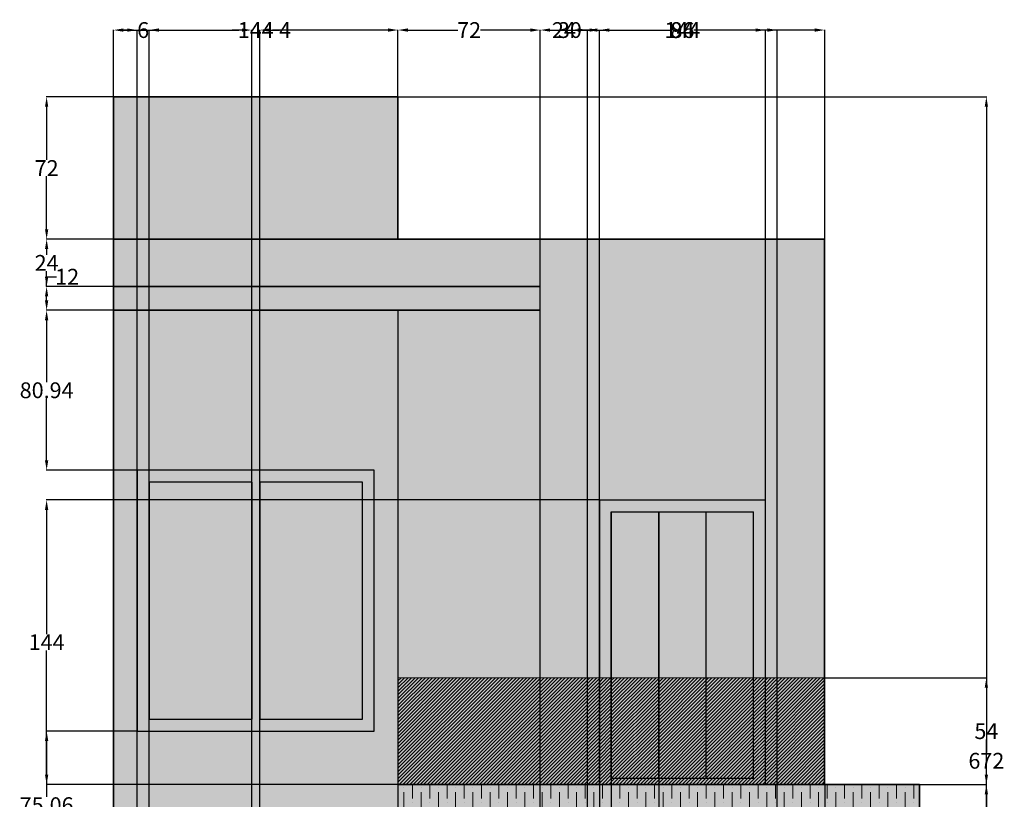
# Model space of a CAD drawing. Units: inches. Extents: x 137 to 641, y 88 to 838.
# Tile 2 of 2: x 142 to 641, y 444 to 838. Entities that reach past the tile are written whole.
import ezdxf

# ---------------------------------------------------------------- set-up
doc = ezdxf.new("R2010")
doc.units = ezdxf.units.IN
doc.header["$MEASUREMENT"] = 0
doc.layers.get('0').update_dxf_attribs({"color": 250})
for name, color, linetype, lineweight in [('A-ANNO-DIMS', 2, 'Continuous', 18), ('A-ELEV-TRIM-PATT', 18, 'Continuous', 13), ('A-FLOR-BALC', 250, 'Continuous', 35), ('A-FLOR-BALC-PATT', 250, 'Continuous', 13), ('A-FLOR-RAIL', 250, 'Continuous', 18), ('A-GLAZ', 250, 'Continuous', 25), ('A-GLAZ-PATT', 250, 'Continuous', 13), ('A-ROOF', 250, 'Continuous', 35), ('A-WALL', 250, 'Continuous', 35), ('A-WALL-CLAD', 250, 'Continuous', 25)]:
    doc.layers.add(name, color=color, linetype=linetype, lineweight=lineweight)
for name, color, linetype, lineweight, true_color in [('A-FLOR-BALC-FILL', 89, 'Continuous', 13, 0x333e19), ('A-FLOR-RAIL-PATT', 251, 'Continuous', 13, 0x636466), ('A-ROOF-PATT', 250, 'Continuous', 13, 0x303030), ('A-WALL-CLAD-FILL', 51, 'Continuous', 13, 0xfff4a4), ('A-WALL-CLAD-PATT', 21, 'Continuous', 13, 0xe2a688), ('A-WALL-PATT', 254, 'Continuous', 13, 0xd7ebd2)]:
    doc.layers.add(name, color=color, linetype=linetype, lineweight=lineweight, true_color=true_color)
doc.styles.get("Standard").update_dxf_attribs({"font": 'arial.ttf'})
doc.dimstyles.get("Standard").update_dxf_attribs({"dimtxt": 8, "dimasz": 5, "dimexe": 0.18, "dimexo": 0.0625, "dimgap": 0.09, "dimtad": 0, "dimtih": 1, "dimtoh": 1, "dimdec": 0, "dimzin": 0, "dimdsep": 46, "dimlunit": 3, "dimtxsty": 'Standard', "dimcen": 0.09, "dimadec": 0, "dimazin": 0, "dimtfac": 1, "dimtdec": 0, "dimtofl": 0, "dimtmove": 0, "dimatfit": 3, "dimfxl": 1, "dimtolj": 1, "dimtzin": 0, "dimarcsym": 0})

# ---------------------------------------------------------------- blocks, each defined once
blk = doc.blocks.new('WIN-FRAME-2L-120X132')
for p, q in [((58, 126), (58, 6)), ((62, 126), (62, 6))]:
    blk.add_line(p, q)
for points in [[(120, 132), (0, 132)], [(0, 132), (0, 0), (120, 0), (120, 132)], [(58, 126), (6, 126)], [(6, 126), (6, 6), (58, 6)], [(62, 6), (114, 6), (114, 126)], [(114, 126), (62, 126)]]:
    blk.add_lwpolyline(points)
blk = doc.blocks.new('*D5')
at = {"layer": 'A-ANNO-DIMS', "color": 0, "lineweight": -2, "transparency": 16777216}
for p, q in [((333.99, 799.23), (631.96, 799.23)), ((631.78, 794.23), (631.78, 467.4)), ((631.78, 132.23), (631.78, 459.05)), ((549.99, 127.23), (631.96, 127.23))]:
    blk.add_line(p, q, dxfattribs=at)
at = {"layer": 'A-ANNO-DIMS', "color": 0, "transparency": 16777216}
for points in [[(630.94, 794.23), (632.61, 794.23), (631.78, 799.23)], [(630.94, 132.23), (632.61, 132.23), (631.78, 127.23)]]:
    blk.add_solid(points, dxfattribs=at)
at = {"layer": 'Defpoints', "color": 0, "transparency": 16777216}
for p in [(333.93, 799.23), (631.78, 799.23), (549.93, 127.23)]:
    blk.add_point(p, dxfattribs=at)
at = {"layer": 'A-ANNO-DIMS', "color": 0, "transparency": 16777216, "insert": (631.78, 463.23), "char_height": 8, "attachment_point": 5}
blk.add_mtext('\\A1;672', dxfattribs=at)
blk = doc.blocks.new('*D6')
at = {"layer": 'A-ANNO-DIMS', "color": 0, "lineweight": -2, "transparency": 16777216}
for p, q in [((189.93, 799.29), (189.93, 833.26)), ((194.93, 833.08), (253.39, 833.08)), ((328.93, 833.08), (270.46, 833.08)), ((333.93, 799.29), (333.93, 833.26))]:
    blk.add_line(p, q, dxfattribs=at)
at = {"layer": 'A-ANNO-DIMS', "color": 0, "transparency": 16777216}
for points in [[(194.93, 833.91), (194.93, 832.25), (189.93, 833.08)], [(328.93, 833.91), (328.93, 832.25), (333.93, 833.08)]]:
    blk.add_solid(points, dxfattribs=at)
at = {"layer": 'Defpoints', "color": 0, "transparency": 16777216}
for p in [(333.93, 833.08), (189.93, 799.23), (333.93, 799.23)]:
    blk.add_point(p, dxfattribs=at)
at = {"layer": 'A-ANNO-DIMS', "color": 0, "transparency": 16777216, "insert": (261.93, 833.08), "char_height": 8, "attachment_point": 5}
blk.add_mtext('\\A1;144', dxfattribs=at)
blk = doc.blocks.new('*D7')
at = {"layer": 'A-ANNO-DIMS', "color": 0, "lineweight": -2, "transparency": 16777216}
for p, q in [((333.93, 799.29), (333.93, 833.26)), ((338.93, 833.08), (364.18, 833.08)), ((400.93, 833.08), (375.67, 833.08)), ((405.93, 703.29), (405.93, 833.26))]:
    blk.add_line(p, q, dxfattribs=at)
at = {"layer": 'A-ANNO-DIMS', "color": 0, "transparency": 16777216}
for points in [[(338.93, 833.91), (338.93, 832.25), (333.93, 833.08)], [(400.93, 833.91), (400.93, 832.25), (405.93, 833.08)]]:
    blk.add_solid(points, dxfattribs=at)
at = {"layer": 'Defpoints', "color": 0, "transparency": 16777216}
for p in [(405.93, 833.08), (333.93, 799.23), (405.93, 703.23)]:
    blk.add_point(p, dxfattribs=at)
at = {"layer": 'A-ANNO-DIMS', "color": 0, "transparency": 16777216, "insert": (369.93, 833.08), "char_height": 8, "attachment_point": 5}
blk.add_mtext('\\A1;72', dxfattribs=at)
blk = doc.blocks.new('*D8')
at = {"layer": 'A-ANNO-DIMS', "color": 0, "lineweight": -2, "transparency": 16777216}
for p, q in [((405.93, 703.29), (405.93, 833.26)), ((410.93, 833.08), (469.39, 833.08)), ((544.93, 833.08), (486.46, 833.08)), ((549.93, 727.29), (549.93, 833.26))]:
    blk.add_line(p, q, dxfattribs=at)
at = {"layer": 'A-ANNO-DIMS', "color": 0, "transparency": 16777216}
for points in [[(410.93, 833.91), (410.93, 832.25), (405.93, 833.08)], [(544.93, 833.91), (544.93, 832.25), (549.93, 833.08)]]:
    blk.add_solid(points, dxfattribs=at)
at = {"layer": 'Defpoints', "color": 0, "transparency": 16777216}
for p in [(549.93, 833.08), (549.93, 727.23), (405.93, 703.23)]:
    blk.add_point(p, dxfattribs=at)
at = {"layer": 'A-ANNO-DIMS', "color": 0, "transparency": 16777216, "insert": (477.93, 833.08), "char_height": 8, "attachment_point": 5}
blk.add_mtext('\\A1;144', dxfattribs=at)
blk = doc.blocks.new('*D10')
at = {"layer": 'A-ANNO-DIMS', "color": 0, "lineweight": -2, "transparency": 16777216}
for p, q in [((201.86, 478.29), (155.9, 478.29)), ((156.08, 473.29), (156.08, 444.93)), ((156.08, 408.23), (156.08, 436.58)), ((333.86, 403.23), (155.9, 403.23))]:
    blk.add_line(p, q, dxfattribs=at)
at = {"layer": 'A-ANNO-DIMS', "color": 0, "transparency": 16777216}
for points in [[(155.24, 473.29), (156.91, 473.29), (156.08, 478.29)], [(155.24, 408.23), (156.91, 408.23), (156.08, 403.23)]]:
    blk.add_solid(points, dxfattribs=at)
at = {"layer": 'Defpoints', "color": 0, "transparency": 16777216}
for p in [(156.08, 478.29), (201.93, 478.29), (333.93, 403.23)]:
    blk.add_point(p, dxfattribs=at)
at = {"layer": 'A-ANNO-DIMS', "color": 0, "transparency": 16777216, "insert": (156.08, 440.76), "char_height": 8, "attachment_point": 5}
blk.add_mtext('\\A1;75.06', dxfattribs=at)
blk = doc.blocks.new('*D11')
at = {"layer": 'A-ANNO-DIMS', "color": 0, "lineweight": -2, "transparency": 16777216}
for p, q in [((189.86, 691.23), (155.9, 691.23)), ((156.08, 686.23), (156.08, 654.93)), ((156.08, 615.29), (156.08, 646.58)), ((201.86, 610.29), (155.9, 610.29))]:
    blk.add_line(p, q, dxfattribs=at)
at = {"layer": 'A-ANNO-DIMS', "color": 0, "transparency": 16777216}
for points in [[(155.24, 686.23), (156.91, 686.23), (156.08, 691.23)], [(155.24, 615.29), (156.91, 615.29), (156.08, 610.29)]]:
    blk.add_solid(points, dxfattribs=at)
at = {"layer": 'Defpoints', "color": 0, "transparency": 16777216}
for p in [(156.08, 691.23), (189.93, 691.23), (201.93, 610.29)]:
    blk.add_point(p, dxfattribs=at)
at = {"layer": 'A-ANNO-DIMS', "color": 0, "transparency": 16777216, "insert": (156.08, 650.76), "char_height": 8, "attachment_point": 5}
blk.add_mtext('\\A1;80.94', dxfattribs=at)
blk = doc.blocks.new('*D12')
at = {"layer": 'A-ANNO-DIMS', "color": 0, "lineweight": -2, "transparency": 16777216}
for p, q in [((156.08, 703.23), (156.08, 708.23)), ((156.08, 708.23), (161.08, 708.23)), ((189.86, 703.23), (155.9, 703.23)), ((156.08, 696.23), (156.08, 698.23)), ((189.86, 691.23), (155.9, 691.23))]:
    blk.add_line(p, q, dxfattribs=at)
at = {"layer": 'A-ANNO-DIMS', "color": 0, "transparency": 16777216}
for points in [[(155.24, 698.23), (156.91, 698.23), (156.08, 703.23)], [(155.24, 696.23), (156.91, 696.23), (156.08, 691.23)]]:
    blk.add_solid(points, dxfattribs=at)
at = {"layer": 'Defpoints', "color": 0, "transparency": 16777216}
for p in [(156.08, 703.23), (189.93, 703.23), (189.93, 691.23)]:
    blk.add_point(p, dxfattribs=at)
at = {"layer": 'A-ANNO-DIMS', "color": 0, "transparency": 16777216, "insert": (166.48, 708.23), "char_height": 8, "attachment_point": 5}
blk.add_mtext('\\A1;12', dxfattribs=at)
blk = doc.blocks.new('*D13')
at = {"layer": 'A-ANNO-DIMS', "color": 0, "lineweight": -2, "transparency": 16777216}
for p, q in [((189.86, 727.23), (155.9, 727.23)), ((156.08, 722.23), (156.08, 719.33)), ((156.08, 708.23), (156.08, 711.12)), ((189.86, 703.23), (155.9, 703.23))]:
    blk.add_line(p, q, dxfattribs=at)
at = {"layer": 'A-ANNO-DIMS', "color": 0, "transparency": 16777216}
for points in [[(155.24, 722.23), (156.91, 722.23), (156.08, 727.23)], [(155.24, 708.23), (156.91, 708.23), (156.08, 703.23)]]:
    blk.add_solid(points, dxfattribs=at)
at = {"layer": 'Defpoints', "color": 0, "transparency": 16777216}
for p in [(156.08, 727.23), (189.93, 727.23), (189.93, 703.23)]:
    blk.add_point(p, dxfattribs=at)
at = {"layer": 'A-ANNO-DIMS', "color": 0, "transparency": 16777216, "insert": (156.08, 715.23), "char_height": 8, "attachment_point": 5}
blk.add_mtext('\\A1;24', dxfattribs=at)
blk = doc.blocks.new('*D14')
at = {"layer": 'A-ANNO-DIMS', "color": 0, "lineweight": -2, "transparency": 16777216}
for p, q in [((189.86, 799.23), (155.9, 799.23)), ((156.08, 794.23), (156.08, 767.33)), ((156.08, 732.23), (156.08, 759.12)), ((189.86, 727.23), (155.9, 727.23))]:
    blk.add_line(p, q, dxfattribs=at)
at = {"layer": 'A-ANNO-DIMS', "color": 0, "transparency": 16777216}
for points in [[(155.24, 794.23), (156.91, 794.23), (156.08, 799.23)], [(155.24, 732.23), (156.91, 732.23), (156.08, 727.23)]]:
    blk.add_solid(points, dxfattribs=at)
at = {"layer": 'Defpoints', "color": 0, "transparency": 16777216}
for p in [(156.08, 799.23), (189.93, 799.23), (189.93, 727.23)]:
    blk.add_point(p, dxfattribs=at)
at = {"layer": 'A-ANNO-DIMS', "color": 0, "transparency": 16777216, "insert": (156.08, 763.23), "char_height": 8, "attachment_point": 5}
blk.add_mtext('\\A1;72', dxfattribs=at)
blk = doc.blocks.new('*D20')
at = {"layer": 'A-ANNO-DIMS', "color": 0, "lineweight": -2, "transparency": 16777216}
for p, q in [((405.93, 175.29), (405.93, 833.26)), ((410.93, 833.08), (412.05, 833.08)), ((424.93, 833.08), (423.8, 833.08)), ((429.93, 175.29), (429.93, 833.26))]:
    blk.add_line(p, q, dxfattribs=at)
at = {"layer": 'A-ANNO-DIMS', "color": 0, "transparency": 16777216}
for points in [[(410.93, 833.91), (410.93, 832.25), (405.93, 833.08)], [(424.93, 833.91), (424.93, 832.25), (429.93, 833.08)]]:
    blk.add_solid(points, dxfattribs=at)
at = {"layer": 'Defpoints', "color": 0, "transparency": 16777216}
for p in [(429.93, 833.08), (405.93, 175.23), (429.93, 175.23)]:
    blk.add_point(p, dxfattribs=at)
at = {"layer": 'A-ANNO-DIMS', "color": 0, "transparency": 16777216, "insert": (417.93, 833.08), "char_height": 8, "attachment_point": 5}
blk.add_mtext('\\A1;24', dxfattribs=at)
blk = doc.blocks.new('*D21')
at = {"layer": 'A-ANNO-DIMS', "color": 0, "lineweight": -2, "transparency": 16777216}
for p, q in [((429.93, 319.29), (429.93, 833.26)), ((434.93, 833.08), (472.11, 833.08)), ((520.93, 833.08), (483.74, 833.08)), ((525.93, 319.29), (525.93, 833.26))]:
    blk.add_line(p, q, dxfattribs=at)
at = {"layer": 'A-ANNO-DIMS', "color": 0, "transparency": 16777216}
for points in [[(434.93, 833.91), (434.93, 832.25), (429.93, 833.08)], [(520.93, 833.91), (520.93, 832.25), (525.93, 833.08)]]:
    blk.add_solid(points, dxfattribs=at)
at = {"layer": 'Defpoints', "color": 0, "transparency": 16777216}
for p in [(525.93, 833.08), (429.93, 319.23), (525.93, 319.23)]:
    blk.add_point(p, dxfattribs=at)
at = {"layer": 'A-ANNO-DIMS', "color": 0, "transparency": 16777216, "insert": (477.93, 833.08), "char_height": 8, "attachment_point": 5}
blk.add_mtext('\\A1;96', dxfattribs=at)
blk = doc.blocks.new('*D30')
at = {"layer": 'A-ANNO-DIMS', "color": 0, "lineweight": -2, "transparency": 16777216}
for p, q in [((196.93, 833.08), (191.93, 833.08)), ((201.93, 199.29), (201.93, 833.26)), ((207.93, 205.29), (207.93, 833.26)), ((212.93, 833.08), (217.93, 833.08))]:
    blk.add_line(p, q, dxfattribs=at)
at = {"layer": 'A-ANNO-DIMS', "color": 0, "transparency": 16777216}
for points in [[(196.93, 833.91), (196.93, 832.25), (201.93, 833.08)], [(212.93, 833.91), (212.93, 832.25), (207.93, 833.08)]]:
    blk.add_solid(points, dxfattribs=at)
at = {"layer": 'Defpoints', "color": 0, "transparency": 16777216}
for p in [(207.93, 833.08), (207.93, 205.23), (201.93, 199.23)]:
    blk.add_point(p, dxfattribs=at)
at = {"layer": 'A-ANNO-DIMS', "color": 0, "transparency": 16777216, "insert": (204.93, 833.08), "char_height": 8, "attachment_point": 5}
blk.add_mtext('\\A1;6', dxfattribs=at)
blk = doc.blocks.new('*D31')
at = {"layer": 'A-ANNO-DIMS', "color": 0, "lineweight": -2, "transparency": 16777216}
for p, q in [((254.93, 833.08), (249.93, 833.08)), ((259.93, 205.29), (259.93, 833.26)), ((263.93, 205.29), (263.93, 833.26)), ((268.93, 833.08), (273.93, 833.08))]:
    blk.add_line(p, q, dxfattribs=at)
at = {"layer": 'A-ANNO-DIMS', "color": 0, "transparency": 16777216}
for points in [[(254.93, 833.91), (254.93, 832.25), (259.93, 833.08)], [(268.93, 833.91), (268.93, 832.25), (263.93, 833.08)]]:
    blk.add_solid(points, dxfattribs=at)
at = {"layer": 'Defpoints', "color": 0, "transparency": 16777216}
for p in [(263.93, 833.08), (259.93, 205.23), (263.93, 205.23)]:
    blk.add_point(p, dxfattribs=at)
at = {"layer": 'A-ANNO-DIMS', "color": 0, "transparency": 16777216, "insert": (276.78, 833.08), "char_height": 8, "attachment_point": 5}
blk.add_mtext('\\A1;4', dxfattribs=at)
blk = doc.blocks.new('*D32')
at = {"layer": 'A-ANNO-DIMS', "color": 0, "lineweight": -2, "transparency": 16777216}
for p, q in [((549.93, 451.17), (549.93, 93.2)), ((597.93, 451.17), (597.93, 93.2)), ((554.93, 93.38), (567.94, 93.38)), ((592.93, 93.38), (579.91, 93.38))]:
    blk.add_line(p, q, dxfattribs=at)
at = {"layer": 'A-ANNO-DIMS', "color": 0, "transparency": 16777216}
for points in [[(554.93, 94.21), (554.93, 92.55), (549.93, 93.38)], [(592.93, 94.21), (592.93, 92.55), (597.93, 93.38)]]:
    blk.add_solid(points, dxfattribs=at)
at = {"layer": 'Defpoints', "color": 0, "transparency": 16777216}
for p in [(549.93, 451.23), (597.93, 451.23), (597.93, 93.38)]:
    blk.add_point(p, dxfattribs=at)
at = {"layer": 'A-ANNO-DIMS', "color": 0, "transparency": 16777216, "insert": (573.93, 93.38), "char_height": 8, "attachment_point": 5}
blk.add_mtext('\\A1;48', dxfattribs=at)
blk = doc.blocks.new('*D33')
at = {"layer": 'A-ANNO-DIMS', "color": 0, "lineweight": -2, "transparency": 16777216}
for p, q in [((597.99, 451.23), (631.96, 451.23)), ((631.78, 446.23), (631.78, 431.4)), ((631.78, 408.23), (631.78, 423.05)), ((597.99, 403.23), (631.96, 403.23))]:
    blk.add_line(p, q, dxfattribs=at)
at = {"layer": 'A-ANNO-DIMS', "color": 0, "transparency": 16777216}
for points in [[(630.94, 446.23), (632.61, 446.23), (631.78, 451.23)], [(630.94, 408.23), (632.61, 408.23), (631.78, 403.23)]]:
    blk.add_solid(points, dxfattribs=at)
at = {"layer": 'Defpoints', "color": 0, "transparency": 16777216}
for p in [(597.93, 451.23), (631.78, 451.23), (597.93, 403.23)]:
    blk.add_point(p, dxfattribs=at)
at = {"layer": 'A-ANNO-DIMS', "color": 0, "transparency": 16777216, "insert": (631.78, 427.23), "char_height": 8, "attachment_point": 5}
blk.add_mtext('\\A1;48', dxfattribs=at)
blk = doc.blocks.new('*D34')
at = {"layer": 'A-ANNO-DIMS', "color": 0, "lineweight": -2, "transparency": 16777216}
for p, q in [((549.99, 505.23), (631.96, 505.23)), ((631.78, 500.23), (631.78, 482.39)), ((631.78, 456.23), (631.78, 474.07)), ((549.99, 451.23), (631.96, 451.23))]:
    blk.add_line(p, q, dxfattribs=at)
at = {"layer": 'A-ANNO-DIMS', "color": 0, "transparency": 16777216}
for points in [[(630.94, 500.23), (632.61, 500.23), (631.78, 505.23)], [(630.94, 456.23), (632.61, 456.23), (631.78, 451.23)]]:
    blk.add_solid(points, dxfattribs=at)
at = {"layer": 'Defpoints', "color": 0, "transparency": 16777216}
for p in [(549.93, 505.23), (631.78, 505.23), (549.93, 451.23)]:
    blk.add_point(p, dxfattribs=at)
at = {"layer": 'A-ANNO-DIMS', "color": 0, "transparency": 16777216, "insert": (631.78, 478.23), "char_height": 8, "attachment_point": 5}
blk.add_mtext('\\A1;54', dxfattribs=at)
blk = doc.blocks.new('*D35')
at = {"layer": 'A-ANNO-DIMS', "color": 0, "lineweight": -2, "transparency": 16777216}
for p, q in [((405.93, 451.29), (405.93, 833.26)), ((410.93, 833.08), (415.12, 833.08)), ((430.93, 833.08), (426.73, 833.08)), ((435.93, 451.29), (435.93, 833.26))]:
    blk.add_line(p, q, dxfattribs=at)
at = {"layer": 'A-ANNO-DIMS', "color": 0, "transparency": 16777216}
for points in [[(410.93, 833.91), (410.93, 832.25), (405.93, 833.08)], [(430.93, 833.91), (430.93, 832.25), (435.93, 833.08)]]:
    blk.add_solid(points, dxfattribs=at)
at = {"layer": 'Defpoints', "color": 0, "transparency": 16777216}
for p in [(435.93, 833.08), (405.93, 451.23), (435.93, 451.23)]:
    blk.add_point(p, dxfattribs=at)
at = {"layer": 'A-ANNO-DIMS', "color": 0, "transparency": 16777216, "insert": (420.93, 833.08), "char_height": 8, "attachment_point": 5}
blk.add_mtext('\\A1;30', dxfattribs=at)
blk = doc.blocks.new('*D36')
at = {"layer": 'A-ANNO-DIMS', "color": 0, "lineweight": -2, "transparency": 16777216}
for p, q in [((435.93, 595.29), (435.93, 833.26)), ((440.93, 833.08), (472.12, 833.08)), ((514.93, 833.08), (483.73, 833.08)), ((519.93, 595.29), (519.93, 833.26))]:
    blk.add_line(p, q, dxfattribs=at)
at = {"layer": 'A-ANNO-DIMS', "color": 0, "transparency": 16777216}
for points in [[(440.93, 833.91), (440.93, 832.25), (435.93, 833.08)], [(514.93, 833.91), (514.93, 832.25), (519.93, 833.08)]]:
    blk.add_solid(points, dxfattribs=at)
at = {"layer": 'Defpoints', "color": 0, "transparency": 16777216}
for p in [(519.93, 833.08), (435.93, 595.23), (519.93, 595.23)]:
    blk.add_point(p, dxfattribs=at)
at = {"layer": 'A-ANNO-DIMS', "color": 0, "transparency": 16777216, "insert": (477.93, 833.08), "char_height": 8, "attachment_point": 5}
blk.add_mtext('\\A1;84', dxfattribs=at)
blk = doc.blocks.new('*D37')
at = {"layer": 'A-ANNO-DIMS', "color": 0, "lineweight": -2, "transparency": 16777216}
for p, q in [((435.86, 595.23), (155.9, 595.23)), ((156.08, 590.23), (156.08, 527.33)), ((156.08, 456.23), (156.08, 519.12)), ((435.86, 451.23), (155.9, 451.23))]:
    blk.add_line(p, q, dxfattribs=at)
at = {"layer": 'A-ANNO-DIMS', "color": 0, "transparency": 16777216}
for points in [[(155.24, 590.23), (156.91, 590.23), (156.08, 595.23)], [(155.24, 456.23), (156.91, 456.23), (156.08, 451.23)]]:
    blk.add_solid(points, dxfattribs=at)
at = {"layer": 'Defpoints', "color": 0, "transparency": 16777216}
for p in [(156.08, 595.23), (435.93, 595.23), (435.93, 451.23)]:
    blk.add_point(p, dxfattribs=at)
at = {"layer": 'A-ANNO-DIMS', "color": 0, "transparency": 16777216, "insert": (156.08, 523.23), "char_height": 8, "attachment_point": 5}
blk.add_mtext('\\A1;144', dxfattribs=at)
blk = doc.blocks.new('*D38')
at = {"layer": 'A-ANNO-DIMS', "color": 0, "lineweight": -2, "transparency": 16777216}
for p, q in [((435.93, 595.17), (435.93, 93.2)), ((441.93, 589.17), (441.93, 93.2)), ((430.93, 93.38), (425.93, 93.38)), ((446.93, 93.38), (451.93, 93.38))]:
    blk.add_line(p, q, dxfattribs=at)
at = {"layer": 'A-ANNO-DIMS', "color": 0, "transparency": 16777216}
for points in [[(430.93, 94.21), (430.93, 92.55), (435.93, 93.38)], [(446.93, 94.21), (446.93, 92.55), (441.93, 93.38)]]:
    blk.add_solid(points, dxfattribs=at)
at = {"layer": 'Defpoints', "color": 0, "transparency": 16777216}
for p in [(435.93, 595.23), (441.93, 589.23), (441.93, 93.38)]:
    blk.add_point(p, dxfattribs=at)
at = {"layer": 'A-ANNO-DIMS', "color": 0, "transparency": 16777216, "insert": (438.93, 93.38), "char_height": 8, "attachment_point": 5}
blk.add_mtext('\\A1;6', dxfattribs=at)
blk = doc.blocks.new('*D39')
at = {"layer": 'A-ANNO-DIMS', "color": 0, "lineweight": -2, "transparency": 16777216}
for p, q in [((441.93, 589.17), (441.93, 93.2)), ((465.93, 589.17), (465.93, 93.2)), ((446.93, 93.38), (448.05, 93.38)), ((460.93, 93.38), (459.8, 93.38))]:
    blk.add_line(p, q, dxfattribs=at)
at = {"layer": 'A-ANNO-DIMS', "color": 0, "transparency": 16777216}
for points in [[(446.93, 94.21), (446.93, 92.55), (441.93, 93.38)], [(460.93, 94.21), (460.93, 92.55), (465.93, 93.38)]]:
    blk.add_solid(points, dxfattribs=at)
at = {"layer": 'Defpoints', "color": 0, "transparency": 16777216}
for p in [(441.93, 589.23), (465.93, 589.23), (465.93, 93.38)]:
    blk.add_point(p, dxfattribs=at)
at = {"layer": 'A-ANNO-DIMS', "color": 0, "transparency": 16777216, "insert": (453.93, 93.38), "char_height": 8, "attachment_point": 5}
blk.add_mtext('\\A1;24', dxfattribs=at)

msp = doc.modelspace()

# ---------------------------------------------------------------- hatches: boundary and pattern name
at = {"layer": 'A-ELEV-TRIM-PATT'}
h = msp.add_hatch(color=256, dxfattribs=at)
h.dxf.hatch_style = 1
h.paths.add_polyline_path([(321.925, 610.288), (201.925, 610.288), (201.925, 478.288), (321.925, 478.288)])
h.paths.add_polyline_path([(263.925, 484.288), (263.925, 604.288), (315.925, 604.288), (315.925, 484.288)], flags=16)
h.paths.add_polyline_path([(259.925, 484.288), (207.925, 484.288), (207.925, 604.288), (259.925, 604.288)], flags=16)
h.paths.add_polyline_path([(321.925, 331.229), (201.925, 331.229), (201.925, 199.229), (321.925, 199.229)])
h.paths.add_polyline_path([(263.925, 325.229), (315.925, 325.229), (315.925, 205.229), (263.925, 205.229)], flags=16)
h.paths.add_polyline_path([(259.925, 325.229), (259.925, 205.229), (207.925, 205.229), (207.925, 325.229)], flags=16)
h = msp.add_hatch(color=256, dxfattribs=at)
h.dxf.hatch_style = 1
h.paths.add_polyline_path([(525.925, 319.229), (429.925, 319.229), (429.925, 175.229), (435.925, 175.229), (435.925, 313.229), (519.925, 313.229), (519.925, 175.229), (525.925, 175.229)])
h.paths.add_polyline_path([(513.925, 280.229), (510.925, 280.229), (510.925, 208.229), (513.925, 208.229), (513.925, 244.229)], flags=17)
h.paths.add_polyline_path([(519.925, 595.229), (435.925, 595.229), (435.925, 505.229), (441.925, 505.229), (441.925, 589.229), (513.925, 589.229), (513.925, 505.229), (519.925, 505.229)])
h.paths.add_polyline_path([(519.925, 505.229), (513.925, 505.229), (513.925, 454.229), (441.925, 454.229), (441.925, 505.229), (435.925, 505.229), (435.925, 451.229), (519.925, 451.229)])
at = {"layer": 'A-FLOR-BALC-FILL'}
msp.add_hatch(color=256, dxfattribs=at).paths.add_polyline_path([(597.925, 451.229), (549.925, 451.229), (333.925, 451.229), (333.925, 403.229), (549.925, 403.229), (597.925, 403.229)])
at = {"layer": 'A-FLOR-BALC-PATT'}
h = msp.add_hatch(dxfattribs=at)
h.set_pattern_fill('ANSI36', color=256, scale=35, angle=45, style=0)
h.paths.add_polyline_path([(597.925, 451.229), (549.925, 451.229), (333.925, 451.229), (333.925, 403.229), (549.925, 403.229), (597.925, 403.229)])
at = {"layer": 'A-FLOR-RAIL-PATT'}
h = msp.add_hatch(dxfattribs=at)
h.set_pattern_fill('ANSI31', color=256, scale=10, style=0)
h.paths.add_polyline_path([(405.925, 505.229), (333.925, 505.229), (333.925, 451.229), (405.925, 451.229)])
h = msp.add_hatch(dxfattribs=at)
h.set_pattern_fill('ANSI31', color=256, scale=10, style=0)
h.paths.add_polyline_path([(435.925, 505.229), (405.925, 505.229), (405.925, 451.229), (435.925, 451.229)])
h = msp.add_hatch(dxfattribs=at)
h.set_pattern_fill('ANSI31', color=256, scale=10, style=0)
h.paths.add_polyline_path([(441.925, 505.229), (435.925, 505.229), (435.925, 451.229), (519.925, 451.229), (519.925, 505.229), (513.925, 505.229), (513.925, 454.229), (441.925, 454.229)])
h = msp.add_hatch(dxfattribs=at)
h.set_pattern_fill('ANSI31', color=256, scale=10, style=0)
h.paths.add_polyline_path([(465.925, 505.229), (441.925, 505.229), (441.925, 454.229), (465.925, 454.229)])
h = msp.add_hatch(dxfattribs=at)
h.set_pattern_fill('ANSI31', color=256, scale=10, style=0)
h.paths.add_polyline_path([(489.925, 505.229), (465.925, 505.229), (465.925, 454.229), (489.925, 454.229)])
h = msp.add_hatch(dxfattribs=at)
h.set_pattern_fill('ANSI31', color=256, scale=10, style=0)
h.paths.add_polyline_path([(513.925, 505.229), (489.925, 505.229), (489.925, 454.229), (513.925, 454.229)])
h = msp.add_hatch(dxfattribs=at)
h.set_pattern_fill('ANSI31', color=256, scale=10, style=0)
h.paths.add_polyline_path([(549.925, 505.229), (519.925, 505.229), (519.925, 451.229), (549.925, 451.229)])
at = {"layer": 'A-GLAZ-PATT'}
h = msp.add_hatch(color=256, dxfattribs=at)
h.set_gradient(color1=(199, 200, 202), color2=(147, 149, 152), rotation=45, name='INVCYLINDER')
h.paths.add_polyline_path([(263.925, 484.288), (315.925, 484.288), (315.925, 604.288), (263.925, 604.288)])
h.paths.add_polyline_path([(259.925, 604.288), (207.925, 604.288), (207.925, 484.288), (259.925, 484.288)])
h = msp.add_hatch(color=256, dxfattribs=at)
h.set_gradient(color1=(199, 200, 202), color2=(147, 149, 152), name='INVCYLINDER')
h.paths.add_polyline_path([(465.925, 589.229), (441.925, 589.229), (441.925, 505.229), (465.925, 505.229)])
h.paths.add_polyline_path([(489.925, 589.229), (465.925, 589.229), (465.925, 505.229), (489.925, 505.229)])
h.paths.add_polyline_path([(513.925, 589.229), (489.925, 589.229), (489.925, 505.229), (513.925, 505.229)])
h.paths.add_polyline_path([(513.925, 505.229), (489.925, 505.229), (489.925, 454.229), (513.925, 454.229)])
h.paths.add_polyline_path([(489.925, 505.229), (465.925, 505.229), (465.925, 454.229), (489.925, 454.229)])
h.paths.add_polyline_path([(465.925, 505.229), (441.925, 505.229), (441.925, 454.229), (465.925, 454.229)])
at = {"layer": 'A-ROOF-PATT'}
h = msp.add_hatch(color=256, dxfattribs=at)
h.dxf.hatch_style = 1
h.paths.add_polyline_path([(333.925, 799.229), (189.925, 799.229), (189.925, 727.229), (333.925, 727.229)])
h.paths.add_polyline_path([(405.925, 703.229), (189.925, 703.229), (189.925, 691.229), (405.925, 691.229)])
at = {"layer": 'A-WALL-CLAD-FILL'}
h = msp.add_hatch(color=256, dxfattribs=at)
h.paths.add_polyline_path([(405.925, 691.229), (333.925, 691.229), (333.925, 505.229), (405.925, 505.229)])
h.paths.add_polyline_path([(405.925, 505.229), (333.925, 505.229), (333.925, 451.229), (405.925, 451.229)])
h.paths.add_polyline_path([(405.925, 403.229), (333.925, 403.229), (333.925, 163.229), (405.925, 163.229)])
at = {"layer": 'A-WALL-CLAD-PATT'}
h = msp.add_hatch(dxfattribs=at)
h.set_pattern_fill('GRAVEL', color=256, scale=15, style=0)
h.set_pattern_definition([(228.01279, (10.8, 15), (-120, -135), [2.01804, -199.78632]), (184.96974, (9.45, 13.5), (180, 15), [3.46302, -342.83887]), (132.51045, (6, 13.2), (150, -165), [2.44182, -241.74049]), (267.27369, (0.15, 9.45), (15, 300), [3.15357, -312.20337]), (292.83365, (0, 6.3), (-75, 180), [3.09232, -306.1406]), (357.27369, (1.2, 3.45), (-300, 15), [3.15357, -312.20337]), (37.69424, (4.35, 3.3), (-195, -150), [4.17043, -412.87273]), (72.25533, (7.65, 5.85), (105, 330), [3.93732, -389.79482]), (121.42957, (8.85, 9.6), (-120, 195), [3.16425, -313.2611]), (175.23636, (7.2, 12.3), (165, -15), [3.61248, -177.01144]), (222.39744, (3.6, 12.6), (-180, -165), [4.67172, -462.50063]), (138.81407, (15, 9.3), (-105, 90), [1.59451, -157.85767]), (171.46923, (13.8, 10.35), (195, -30), [3.03355, -300.32267]), (225, (10.8, 10.8), (-2e-15, -15), [2.12132, -19.0919]), (203.1986, (9.75, 12.6), (75, 30), [1.14237, -113.09423]), (291.8014, (8.7, 12.15), (-15, 45), [1.61555, -79.16193]), (30.96376, (9.3, 10.65), (45, 30), [2.62393, -84.84034]), (161.56505, (11.55, 12), (30, -15), [1.89736, -45.5368]), (16.38954, (0, 12.15), (150, 45), [2.658, -263.14268]), (70.34618, (2.55, 12.9), (-60, -165), [2.22991, -220.76112]), (293.1986, (11.55, 15), (-30, 75), [2.28472, -111.95187]), (343.61046, (12.45, 12.9), (-150, 45), [2.658, -263.14268]), (339.44395, (0, 2.85), (-75, 30), [2.5632, -125.59686]), (294.77514, (2.4, 1.95), (-75, 165), [2.14767, -212.61965]), (66.8014, (11.7, 0), (30, 75), [2.28472, -111.95187]), (17.35402, (12.6, 2.1), (-195, -60), [2.51446, -248.93135]), (69.44395, (4.35, 0), (-30, -75), [1.2816, -126.87846]), (101.30993, (10.8, 0), (-15, 60), [0.76485, -75.72044]), (165.96376, (10.65, 0.75), (45, -15), [3.09233, -58.75426]), (186.00901, (7.65, 1.5), (150, 15), [2.86575, -283.70885]), (303.69007, (9.3, 9.3), (-15, 30), [2.16333, -51.91994]), (353.15723, (10.5, 7.5), (255, -30), [3.77691, -373.91344]), (60.9454, (14.25, 7.05), (-60, -105), [1.54434, -152.89011]), (90, (15, 8.4), (-15, 15), [0.9, -14.1]), (120.25644, (7.35, 1.95), (60, -105), [2.08386, -206.3028]), (48.01279, (6.3, 3.75), (120, 135), [4.03608, -197.76828]), (0, (9, 6.75), (15, 15), [3.9, -11.1]), (325.30485, (12.9, 6.75), (150, -105), [2.3717, -234.79911]), (254.0546, (14.85, 5.4), (-15, -60), [2.18403, -107.01762]), (207.645975, (14.25, 3.3), (-285, -150), [3.55598, -352.04211]), (175.42608, (11.1, 1.65), (-195, 15), [3.76199, -372.4361])])
h.paths.add_polyline_path([(405.925, 691.229), (333.925, 691.229), (333.925, 505.229), (405.925, 505.229)])
h.paths.add_polyline_path([(405.925, 505.229), (333.925, 505.229), (333.925, 451.229), (405.925, 451.229)])
h.paths.add_polyline_path([(405.925, 403.229), (333.925, 403.229), (333.925, 163.229), (405.925, 163.229)])
at = {"layer": 'A-WALL-PATT'}
h = msp.add_hatch(color=256, dxfattribs=at)
h.paths.add_polyline_path([(549.925, 727.229), (189.925, 727.229), (189.925, 703.229), (405.925, 703.229), (405.925, 505.229), (435.925, 505.229), (435.925, 595.229), (519.925, 595.229), (519.925, 505.229), (549.925, 505.229)])
h.paths.add_polyline_path([(549.925, 505.229), (519.925, 505.229), (519.925, 451.229), (549.925, 451.229)])
h.paths.add_polyline_path([(435.925, 505.229), (405.925, 505.229), (405.925, 451.229), (435.925, 451.229)])
h = msp.add_hatch(color=256, dxfattribs=at)
h.dxf.hatch_style = 1
h.paths.add_polyline_path([(189.925, 163.229), (333.925, 163.229), (333.925, 691.229), (189.925, 691.229)])
h.paths.add_polyline_path([(201.925, 478.288), (201.925, 610.288), (321.925, 610.288), (321.925, 478.288)], flags=16)
h.paths.add_polyline_path([(207.925, 484.288), (207.925, 604.288), (259.925, 604.288), (259.925, 484.288)], flags=0)
h.paths.add_polyline_path([(263.925, 484.288), (263.925, 604.288), (315.925, 604.288), (315.925, 484.288)], flags=0)
h.paths.add_polyline_path([(321.925, 331.229), (321.925, 199.229), (201.925, 199.229), (201.925, 331.229)], flags=16)
h.paths.add_polyline_path([(259.925, 325.229), (259.925, 205.229), (207.925, 205.229), (207.925, 325.229)], flags=0)
h.paths.add_polyline_path([(263.925, 325.229), (315.925, 325.229), (315.925, 205.229), (263.925, 205.229)], flags=0)

# ---------------------------------------------------------------- linework, layer by layer
at = {"layer": 'A-FLOR-BALC'}
for p, q in [((549.925, 451.229), (333.925, 451.229)), ((549.925, 451.229), (597.925, 451.229)), ((597.925, 451.229), (597.925, 403.229))]:
    msp.add_line(p, q, dxfattribs=at)
at = {"layer": 'A-FLOR-RAIL'}
msp.add_line((549.925, 505.229), (333.925, 505.229), dxfattribs=at)
at = {"layer": 'A-GLAZ'}
for p, q in [((435.925, 451.229), (435.925, 595.229)), ((435.925, 595.229), (519.925, 595.229)), ((519.925, 451.229), (519.925, 595.229)), ((441.925, 589.229), (513.925, 589.229)), ((441.925, 454.229), (441.925, 589.229)), ((465.925, 454.229), (465.925, 589.229)), ((489.925, 454.229), (489.925, 589.229)), ((513.925, 454.229), (513.925, 589.229)), ((513.925, 454.229), (441.925, 454.229))]:
    msp.add_line(p, q, dxfattribs=at)
at = {"layer": 'A-ROOF'}
for p, q in [((189.925, 727.229), (189.925, 799.229)), ((333.925, 799.229), (189.925, 799.229)), ((333.925, 727.229), (333.925, 799.229)), ((405.925, 703.229), (189.925, 703.229)), ((405.925, 691.229), (189.925, 691.229))]:
    msp.add_line(p, q, dxfattribs=at)
at = {"layer": 'A-WALL'}
for p, q in [((549.925, 727.229), (189.925, 727.229)), ((189.925, 727.229), (189.925, 127.229)), ((549.925, 451.229), (549.925, 727.229))]:
    msp.add_line(p, q, dxfattribs=at)
at = {"layer": 'A-WALL-CLAD'}
for p, q in [((405.925, 451.229), (405.925, 703.229)), ((333.925, 691.229), (333.925, 163.229))]:
    msp.add_line(p, q, dxfattribs=at)

# ---------------------------------------------------------------- block references
at = {"layer": 'A-GLAZ'}
msp.add_blockref('WIN-FRAME-2L-120X132', (201.925, 478.288), dxfattribs=at)

# ---------------------------------------------------------------- dimensions: what is measured, and where the dimension line sits
at = {"layer": 'A-ANNO-DIMS'}
for base, p1, p2, picture, middle in [((333.925, 833.079), (189.925, 799.229), (333.925, 799.229), '*D6', (261.925, 833.079)), ((207.925, 833.079), (201.925, 199.229), (207.925, 205.229), '*D30', (204.925, 833.079)), ((263.925, 833.079), (259.925, 205.229), (263.925, 205.229), '*D31', (276.782, 833.079)), ((405.925, 833.079), (333.925, 799.229), (405.925, 703.229), '*D7', (369.925, 833.079)), ((549.925, 833.079), (405.925, 703.229), (549.925, 727.229), '*D8', (477.925, 833.079)), ((429.925, 833.079), (405.925, 175.229), (429.925, 175.229), '*D20', (417.925, 833.079)), ((435.925, 833.079), (405.925, 451.229), (435.925, 451.229), '*D35', (420.925, 833.079)), ((525.925, 833.079), (429.925, 319.229), (525.925, 319.229), '*D21', (477.925, 833.079)), ((519.925, 833.079), (435.925, 595.229), (519.925, 595.229), '*D36', (477.925, 833.079)), ((441.925, 93.379), (435.925, 595.229), (441.925, 589.229), '*D38', (438.925, 93.379)), ((465.925, 93.379), (441.925, 589.229), (465.925, 589.229), '*D39', (453.925, 93.379)), ((597.925, 93.379), (549.925, 451.229), (597.925, 451.229), '*D32', (573.925, 93.379))]:
    dim = msp.add_linear_dim(base=base, p1=p1, p2=p2, dimstyle='Standard', override={"dimdec": 0, "dimlfac": 1, "dimrnd": 0, "dimzin": 0, "dimdsep": 46, "dimlunit": 2}, dxfattribs=at)
    dim.commit()
    dim.dimension.update_dxf_attribs({"geometry": picture, "text_midpoint": middle})
for base, p1, p2, override, picture, middle in [((156.075, 799.229), (189.925, 727.229), (189.925, 799.229), {"dimdec": 0, "dimlfac": 1, "dimrnd": 0, "dimzin": 0, "dimdsep": 46, "dimlunit": 2}, '*D14', (156.075, 763.229)), ((631.775, 799.229), (549.925, 127.229), (333.925, 799.229), {"dimdec": 0, "dimlfac": 1, "dimrnd": 0, "dimzin": 0, "dimdsep": 46, "dimlunit": 2}, '*D5', (631.775, 463.229)), ((156.075, 727.229), (189.925, 703.229), (189.925, 727.229), {"dimdec": 0, "dimlfac": 1, "dimrnd": 0, "dimzin": 0, "dimdsep": 46, "dimlunit": 2}, '*D13', (156.075, 715.229)), ((156.075, 703.229), (189.925, 691.229), (189.925, 703.229), {"dimdec": 0, "dimlfac": 1, "dimrnd": 0, "dimzin": 0, "dimdsep": 46, "dimlunit": 2}, '*D12', (166.478, 708.229)), ((156.075, 691.229), (201.925, 610.288), (189.925, 691.229), {"dimdec": 2, "dimlfac": 1, "dimrnd": 0, "dimzin": 0, "dimdsep": 46, "dimlunit": 2}, '*D11', (156.075, 650.758)), ((156.075, 595.229), (435.925, 451.229), (435.925, 595.229), {"dimdec": 0, "dimlfac": 1, "dimrnd": 0, "dimzin": 0, "dimdsep": 46, "dimlunit": 2}, '*D37', (156.075, 523.229)), ((631.775, 505.229), (549.925, 451.229), (549.925, 505.229), {"dimdec": 0, "dimlfac": 1, "dimrnd": 0, "dimzin": 0, "dimdsep": 46, "dimlunit": 2}, '*D34', (631.775, 478.229)), ((156.075, 478.288), (333.925, 403.229), (201.925, 478.288), {"dimdec": 2, "dimlfac": 1, "dimrnd": 0, "dimzin": 0, "dimdsep": 46, "dimlunit": 2}, '*D10', (156.075, 440.758)), ((631.775, 451.229), (597.925, 403.229), (597.925, 451.229), {"dimdec": 0, "dimlfac": 1, "dimrnd": 0, "dimzin": 0, "dimdsep": 46, "dimlunit": 2}, '*D33', (631.775, 427.229))]:
    dim = msp.add_linear_dim(base=base, p1=p1, p2=p2, angle=90, dimstyle='Standard', override=override, dxfattribs=at)
    dim.commit()
    dim.dimension.update_dxf_attribs({"geometry": picture, "text_midpoint": middle})

doc.saveas('drawing.dxf')
